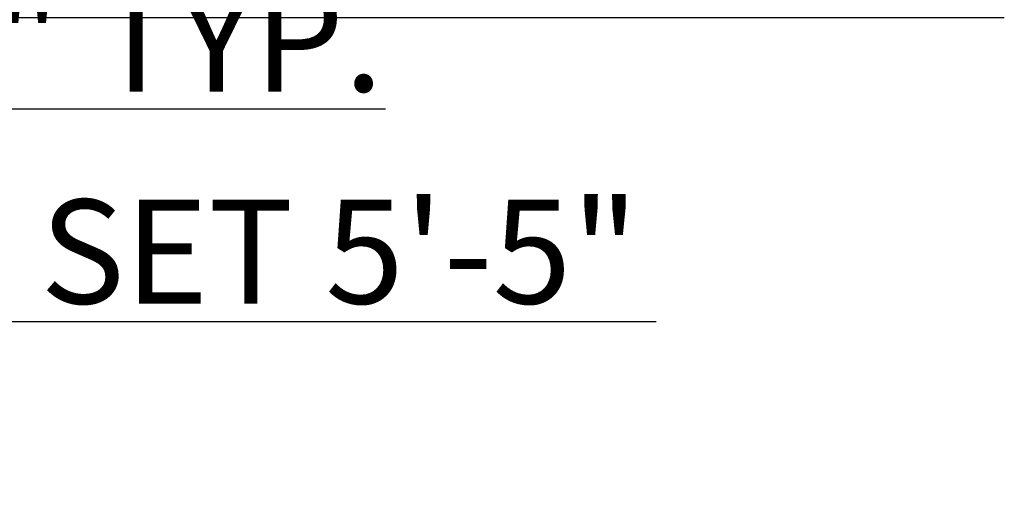
# Model space of a CAD drawing. Units: inches. Extents: x -584 to 444, y 228 to 1001.
# Tile 4 of 5: x 217 to 444, y 534 to 647. Entities that reach past the tile are written whole.
import ezdxf

# ---------------------------------------------------------------- set-up
doc = ezdxf.new("R2010")
doc.units = ezdxf.units.IN
doc.layers.add('A-ANNO-DIMS', color=2, linetype='Continuous', lineweight=18)
doc.styles.get("Standard").update_dxf_attribs({"font": 'arial.ttf'})
doc.dimstyles.new('ISO-25', dxfattribs={"dimtxt": 24, "dimasz": 24, "dimexe": 1.25, "dimexo": 0.625, "dimtad": 1, "dimdec": 1, "dimlunit": 3, "dimtxsty": 'Standard', "dimcen": 2.5, "dimadec": 0, "dimazin": 0, "dimtfac": 1, "dimtdec": 1, "dimtmove": 0, "dimatfit": 3, "dimfxl": 1, "dimarcsym": 0})

# ---------------------------------------------------------------- blocks, each defined once
blk = doc.blocks.new('*D12')
at = {"layer": 'A-ANNO-DIMS', "color": 0, "lineweight": -2, "transparency": 16777216}
for p, q in [((96.86, 617.66), (96.86, 627.29)), ((105.86, 617.66), (105.86, 627.29)), ((72.86, 626.04), (48.86, 626.04)), ((96.86, 626.04), (105.86, 626.04)), ((129.86, 626.04), (301.4, 626.04))]:
    blk.add_line(p, q, dxfattribs=at)
at = {"layer": 'A-ANNO-DIMS', "color": 0, "transparency": 16777216}
for points in [[(72.86, 630.04), (72.86, 622.04), (96.86, 626.04)], [(129.86, 630.04), (129.86, 622.04), (105.86, 626.04)]]:
    blk.add_solid(points, dxfattribs=at)
at = {"layer": 'Defpoints', "color": 0, "transparency": 16777216}
for p in [(105.86, 626.04), (96.86, 617.04), (105.86, 617.04)]:
    blk.add_point(p, dxfattribs=at)
at = {"layer": 'A-ANNO-DIMS', "color": 0, "transparency": 16777216, "insert": (227.63, 638.92), "char_height": 24, "attachment_point": 5}
blk.add_mtext('0\'-9" TYP.', dxfattribs=at)
blk = doc.blocks.new('*D17')
at = {"layer": 'A-ANNO-DIMS', "color": 0, "lineweight": -2, "transparency": 16777216}
for p, q in [((-20.14, 651.91), (-20.14, 645.89)), ((15.86, 651.91), (15.86, 645.89)), ((-44.14, 647.14), (-68.14, 647.14)), ((-20.14, 647.14), (15.86, 647.14)), ((39.86, 647.14), (444.11, 647.14))]:
    blk.add_line(p, q, dxfattribs=at)
at = {"layer": 'A-ANNO-DIMS', "color": 0, "transparency": 16777216}
for points in [[(-44.14, 651.14), (-44.14, 643.14), (-20.14, 647.14)], [(39.86, 651.14), (39.86, 643.14), (15.86, 647.14)]]:
    blk.add_solid(points, dxfattribs=at)
at = {"layer": 'Defpoints', "color": 0, "transparency": 16777216}
for p in [(-20.14, 652.54), (15.86, 652.54), (15.86, 647.14)]:
    blk.add_point(p, dxfattribs=at)
at = {"layer": 'A-ANNO-DIMS', "color": 0, "transparency": 16777216, "insert": (253.99, 660.19), "char_height": 24, "attachment_point": 5}
blk.add_mtext('SWING DOOR 3\'-0" TYP.', dxfattribs=at)
blk = doc.blocks.new('*D25')
at = {"layer": 'A-ANNO-DIMS', "color": 0, "lineweight": -2, "transparency": 16777216}
for p, q in [((9.69, 586.14), (9.69, 575.76)), ((74.75, 586.14), (74.75, 575.76)), ((33.69, 577.01), (50.75, 577.01)), ((74.75, 577.01), (363.79, 577.01))]:
    blk.add_line(p, q, dxfattribs=at)
at = {"layer": 'A-ANNO-DIMS', "color": 0, "transparency": 16777216}
for points in [[(33.69, 581.01), (33.69, 573.01), (9.69, 577.01)], [(50.75, 581.01), (50.75, 573.01), (74.75, 577.01)]]:
    blk.add_solid(points, dxfattribs=at)
at = {"layer": 'Defpoints', "color": 0, "transparency": 16777216}
for p in [(9.69, 586.77), (74.75, 586.77), (74.75, 577.01)]:
    blk.add_point(p, dxfattribs=at)
at = {"layer": 'A-ANNO-DIMS', "color": 0, "transparency": 16777216, "insert": (231.27, 590.04), "char_height": 24, "attachment_point": 5}
blk.add_mtext('DINING SET 5\'-5"', dxfattribs=at)

msp = doc.modelspace()

# ---------------------------------------------------------------- dimensions: what is measured, and where the dimension line sits
at = {"layer": 'A-ANNO-DIMS'}
for base, p1, p2, text, picture, middle in [((15.86, 647.14), (-20.14, 652.54), (15.86, 652.54), 'SWING DOOR <> TYP.', '*D17', (253.99, 660.19)), ((105.86, 626.04), (96.86, 617.04), (105.86, 617.04), '<> TYP.', '*D12', (227.63, 638.92)), ((74.75, 577.01), (9.69, 586.77), (74.75, 586.77), 'DINING SET <>', '*D25', (231.27, 590.04))]:
    dim = msp.add_linear_dim(base=base, p1=p1, p2=p2, text=text, dimstyle='ISO-25', override={"dimdec": 1, "dimlfac": 1, "dimrnd": 0, "dimzin": 1, "dimdsep": 46, "dimlunit": 4, "dimfrac": 2}, dxfattribs=at)
    dim.commit()
    dim.dimension.update_dxf_attribs({"geometry": picture, "text_midpoint": middle})

doc.saveas('drawing.dxf')
